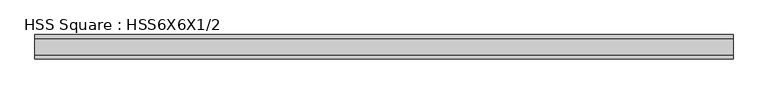
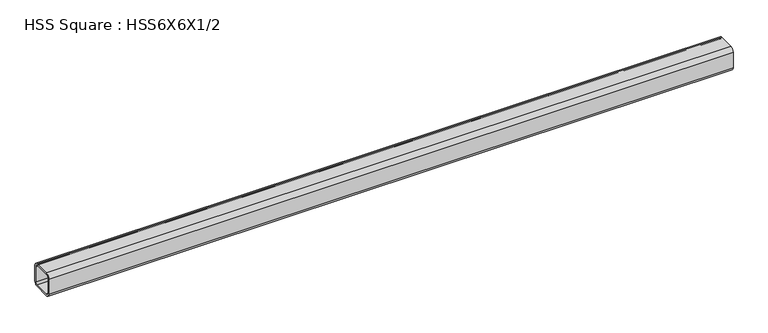
"""IFC4 building model written with IfcOpenShell, lengths in millimetres: member geometry, HSS Square : HSS6X6X1/2."""

from ifc_helpers import new_model, si_unit, point, frame, frame_2d, origin, place, context, project, spatial, polyline, circle_curve, trimmed, segment, composite_curve, outline, extrude, source, transform, mapped, element, save


def hss_square_hss6x6x1_2_f7a49a43(model_context):
    return source(origin(), model_context, "Body", "SweptSolid", [
        extrude(outline(composite_curve([segment(polyline([(76.2, 50.8), (76.2, -50.8)]), True, "CONTINUOUS"), segment(trimmed(circle_curve(frame_2d((50.8, -50.8)), 25.4), [point((76.2, -50.8))], [point((50.8, -76.2))], False, "CARTESIAN"), True, "CONTINUOUS"), segment(polyline([(50.8, -76.2), (-50.8, -76.2)]), True, "CONTINUOUS"), segment(trimmed(circle_curve(frame_2d((-50.8, -50.8)), 25.4), [point((-50.8, -76.2))], [point((-76.2, -50.8))], False, "CARTESIAN"), True, "CONTINUOUS"), segment(polyline([(-76.2, -50.8), (-76.2, 50.8)]), True, "CONTINUOUS"), segment(trimmed(circle_curve(frame_2d((-50.8, 50.8)), 25.4), [point((-76.2, 50.8))], [point((-50.8, 76.2))], False, "CARTESIAN"), True, "CONTINUOUS"), segment(polyline([(-50.8, 76.2), (50.8, 76.2)]), True, "CONTINUOUS"), segment(trimmed(circle_curve(frame_2d((50.8, 50.8)), 25.4), [point((50.8, 76.2))], [point((76.2, 50.8))], False, "CARTESIAN"), True, "CONTINUOUS")], self_intersect=False), holes=[composite_curve([segment(trimmed(circle_curve(frame_2d((-50.8, 50.8)), 12.7), [point((-50.8, 63.5))], [point((-63.5, 50.8))], True, "CARTESIAN"), True, "CONTINUOUS"), segment(polyline([(-63.5, 50.8), (-63.5, -50.8)]), True, "CONTINUOUS"), segment(trimmed(circle_curve(frame_2d((-50.8, -50.8)), 12.7), [point((-63.5, -50.8))], [point((-50.8, -63.5))], True, "CARTESIAN"), True, "CONTINUOUS"), segment(polyline([(-50.8, -63.5), (50.8, -63.5)]), True, "CONTINUOUS"), segment(trimmed(circle_curve(frame_2d((50.8, -50.8)), 12.7), [point((50.8, -63.5))], [point((63.5, -50.8))], True, "CARTESIAN"), True, "CONTINUOUS"), segment(polyline([(63.5, -50.8), (63.5, 50.8)]), True, "CONTINUOUS"), segment(trimmed(circle_curve(frame_2d((50.8, 50.8)), 12.7), [point((63.5, 50.8))], [point((50.8, 63.5))], True, "CARTESIAN"), True, "CONTINUOUS"), segment(polyline([(50.8, 63.5), (-50.8, 63.5)]), True, "CONTINUOUS")], self_intersect=False)]), frame((-2223.7065373, 0.0, 0.0), z_axis=(1.0, 0.0, 0.0), x_axis=(0.0, 1.0, 0.0)), (0.0, 0.0, 1.0), 4352.793108),
    ])


if __name__ == "__main__":
    model = new_model("IFC4")
    model_context = context("Model", 3, world=origin())
    ifc_project = project(units=[si_unit("LENGTHUNIT", "METRE", prefix="MILLI")], contexts=[model_context])
    site = spatial("IfcSite", under=ifc_project)
    building = spatial("IfcBuilding", under=site)
    placement = place(None, origin())
    hss_square_hss6x6x1_2_shape = hss_square_hss6x6x1_2_f7a49a43(model_context)
    element("IfcMember", 1, ObjectType="HSS Square : HSS6X6X1/2", at=placement, inside=building, context=model_context, shape_type="MappedRepresentation", body=[
        mapped(hss_square_hss6x6x1_2_shape, transform((0.0, 0.0, 0.0), x_axis=(1.0, 0.0, 0.0), y_axis=(0.0, 1.0, 0.0), z_axis=(0.0, 0.0, 1.0))),
    ])
    save(model, "model.ifc")

# Revit data of these elements
# Type "HSS Square : HSS6X6X1/2"
#   Section Name Key = "HSS 6X6X1/2"
#   Assembly Code = "B10"
#   Width = 6.000"
#   Wall Nominal Thickness = 0.500"
#   Wall Design Thickness = 0.465"
#   Torsional Moment of Inertia = 81.10 in⁴
#   Torsional Modulus = 28.10 in³
#   Section Area = 9.74 in²
#   Plastic Modulus weak axis = 19.80 in³
#   Plastic Modulus strong axis = 19.80 in³
#   Outer Fillet = 1.000"
#   Nominal Weight = 35.24 lbf/ft
#   Moment of Inertia weak axis = 48.30 in⁴
#   Moment of Inertia strong axis = 48.30 in⁴
#   Inner Fillet = 0.500"
#   Height = 6.000"
#   Elastic Modulus weak axis = 16.10 in³
#   Elastic Modulus strong axis = 16.10 in³
#   Centroid Vertical = 3.000"
#   Centroid Horizontal = 3.000"
#   Length [instance default] = 5' - 0"
#   Structural Material [instance default] = Steel ASTM A500, Grade B, Rectangular and Square
#   Principal Axes Angle = 0
# Element 1 (IfcMember, "HSS Square : HSS6X6X1/2")
#   Structural Material = Steel ASTM A992
#   Materials on its faces: "Steel ASTM A992"
# Materials
#   "Steel ASTM A500, Grade B, Rectangular and Square": class "Metal", colour RGB 199 199 199, transparency 0, Description = "Carbon steel", Cost = 0
#   "Steel ASTM A992": class "Metal", colour RGB 199 199 199, transparency 0, Description = "Structural steel 50ksi", Cost = 0
